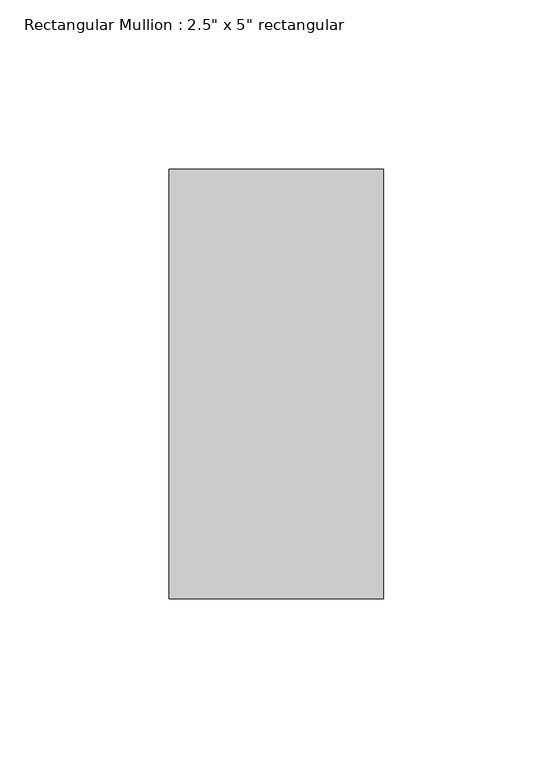
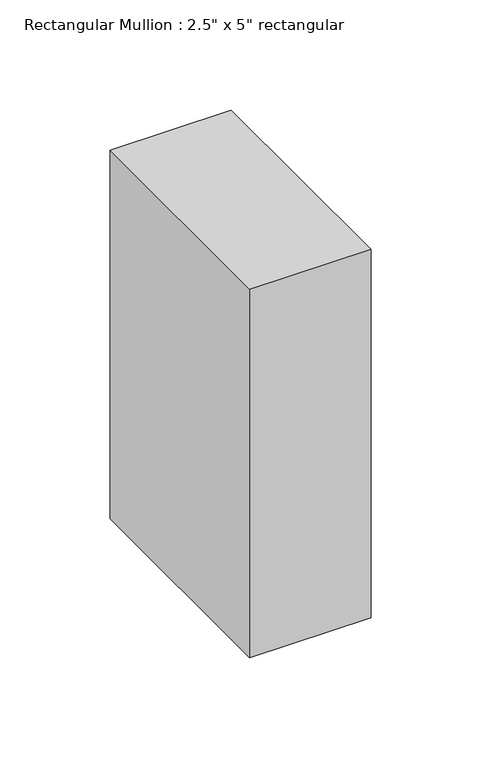
"""IFC4 building model written with IfcOpenShell, lengths in millimetres: member geometry."""

from ifc_helpers import new_model, si_unit, frame, origin, place, context, project, spatial, polyline, outline, extrude, source, transform, mapped, element, save


def member_e8ffc670(model_context):
    return source(origin(), model_context, "Body", "SweptSolid", [
        extrude(outline(polyline([(0.0, 63.5), (0.0, -63.5), (-63.5, -63.5), (-63.5, 63.5), (0.0, 63.5)])), frame((0.0, 0.0, -204.47), z_axis=(0.0, 0.0, 1.0), x_axis=(1.0, 0.0, 0.0)), (0.0, 0.0, 1.0), 204.47),
    ])


if __name__ == "__main__":
    model = new_model("IFC4")
    model_context = context("Model", 3, world=origin())
    ifc_project = project(units=[si_unit("LENGTHUNIT", "METRE", prefix="MILLI")], contexts=[model_context])
    site = spatial("IfcSite", under=ifc_project)
    building = spatial("IfcBuilding", under=site)
    placement = place(None, origin())
    member_shape = member_e8ffc670(model_context)
    element("IfcMember", 1, ObjectType="Rectangular Mullion : 2.5\" x 5\" rectangular", at=placement, inside=building, context=model_context, shape_type="MappedRepresentation", body=[
        mapped(member_shape, transform((0.0, 0.0, 0.0), x_axis=(1.0, 0.0, 0.0), y_axis=(0.0, 1.0, 0.0), z_axis=(0.0, 0.0, 1.0))),
    ])
    save(model, "model.ifc")

# Revit data of these elements
# Type "Rectangular Mullion : 2.5\" x 5\" rectangular"
#   built-in parameter 1007304 = 0.416667 (stored number, unit not read)
#   built-in parameter 1007301 = 0.104167 (stored number, unit not read)
#   built-in parameter 1007300 = 0.104167 (stored number, unit not read)
# Element 1 (IfcMember, "Rectangular Mullion : 2.5\" x 5\" rectangular")
#   Materials on its faces: "Aluminum"
# Materials
#   "Aluminum": class "Metal", colour RGB 247 247 247, transparency 0, Description = "Aluminum 6061", Cost = 0
